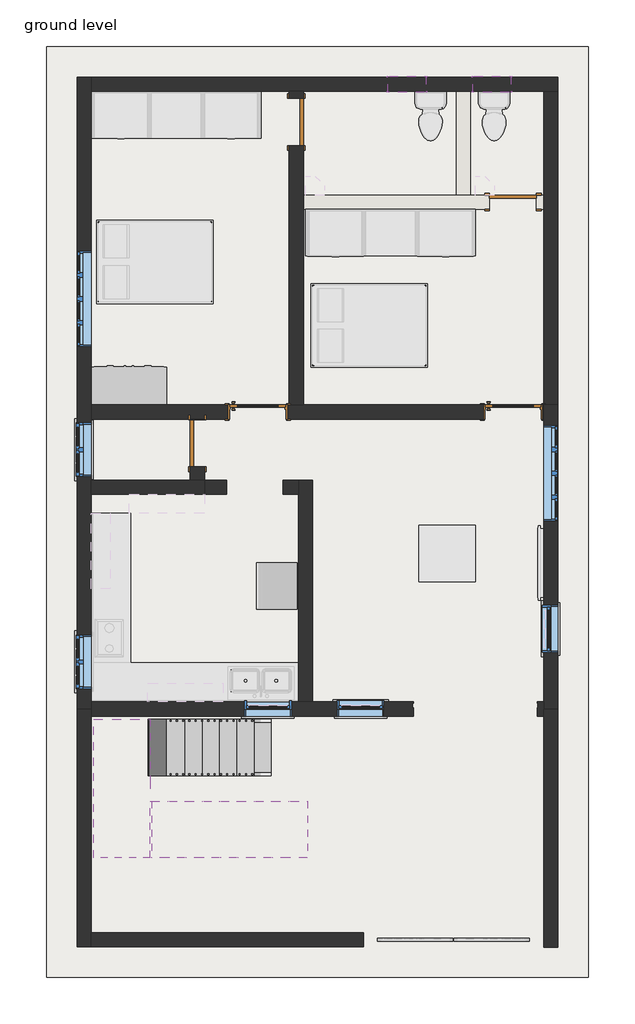
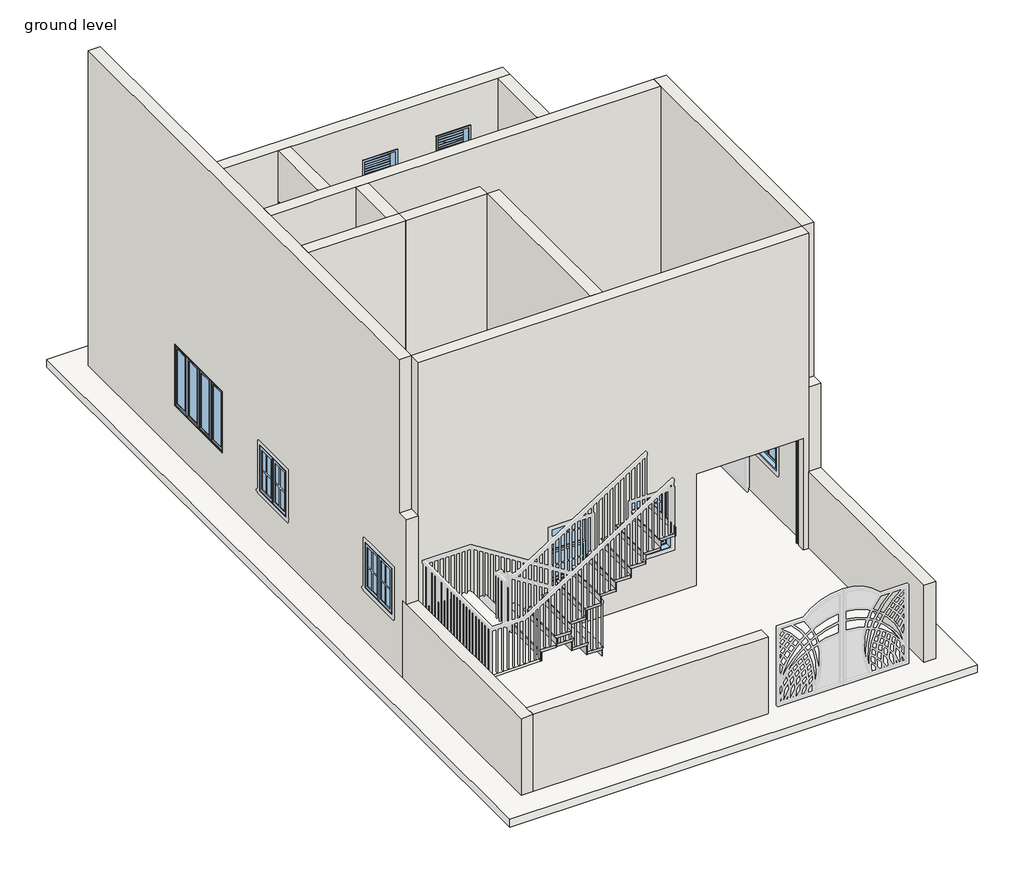
# One storey, part 1 of 3: 16 walls, 9 windows, 5 doors, 2 slabs, 2 stair flights.
"""IFC4 building model written with IfcOpenShell, lengths in millimetres."""

from ifc_helpers import new_model, si_unit, point, frame, origin, place, context, project, spatial, polyline, ellipse_curve, trimmed, outline, extrude, faceted_brep, transform, mapped, element, save
from ifc_brep_helpers import plane_surface, extruded_surface, advanced_brep
from components import door_3b97b8e7, door_bb98abfd, door_5e1232af, non_monolithic_landing_62f4187a, stair_flight_1669251e, stair_flight_fc52eaa6, window_339605e1, window_cf6260c5, window_d400040f, window_f2d8fef0

model = new_model("IFC4")

# Units and contexts
model_context = context("Model", 3, world=origin())
ifc_project = project(units=[si_unit("LENGTHUNIT", "METRE", prefix="MILLI")], contexts=[model_context])

# Site, building, storey
site = spatial("IfcSite", under=ifc_project)
building = spatial("IfcBuilding", under=site)
storey = spatial("IfcBuildingStorey", under=building, Name="ground level", Elevation=609.6)

# Doors
placement = place(None, origin())
door_shape = door_3b97b8e7(model_context)
element("IfcDoor", 1, ObjectType="Door-Interior-Single-1_Panel-Wood : 36\" x 84\"", at=placement, inside=storey, context=model_context, shape_type="MappedRepresentation", body=[
    mapped(door_shape, transform((31303.3316163, 14251.2730552, 609.6), x_axis=(1.0, 0.0, 0.0), y_axis=(0.0, 1.0, 0.0), z_axis=(0.0, 0.0, 1.0))),
])
element("IfcDoor", 2, ObjectType="Door-Interior-Single-1_Panel-Wood : 36\" x 84\"", at=placement, inside=storey, context=model_context, shape_type="MappedRepresentation", body=[
    mapped(door_shape, transform((35430.8316163, 14251.2730552, 609.6), x_axis=(1.0, 0.0, 0.0), y_axis=(0.0, 1.0, 0.0), z_axis=(0.0, 0.0, 1.0))),
])
door_2_shape = door_bb98abfd(model_context)
element("IfcDoor", 3, ObjectType="Single-Flush : 30\" x 84\"", at=placement, inside=storey, context=model_context, shape_type="MappedRepresentation", body=[
    mapped(door_2_shape, transform((30325.4316163, 13740.0980552, 609.6), x_axis=(0.0, 1.0, 0.0), y_axis=(-1.0, 0.0, 0.0), z_axis=(0.0, 0.0, 1.0))),
])
element("IfcDoor", 4, ObjectType="Single-Flush : 30\" x 84\"", at=placement, inside=storey, context=model_context, shape_type="MappedRepresentation", body=[
    mapped(door_2_shape, transform((35430.8316163, 17638.9980552, 609.6), x_axis=(1.0, 0.0, 0.0), y_axis=(0.0, 1.0, 0.0), z_axis=(0.0, 0.0, 1.0))),
])
door_3_shape = door_5e1232af(model_context)
element("IfcDoor", 5, ObjectType="Single-Flush : 30\" x 84\"", at=placement, inside=storey, context=model_context, shape_type="MappedRepresentation", body=[
    mapped(door_3_shape, transform((31925.6316163, 18934.3980552, 609.6), x_axis=(0.0, 1.0, 0.0), y_axis=(-1.0, 0.0, 0.0), z_axis=(0.0, 0.0, 1.0))),
])

# Slabs
element("IfcSlab", 6, ObjectType="Generic - 12\" 2", at=placement, inside=storey, context=model_context, shape_type="SweptSolid", body=[
    extrude(outline(polyline([(36650.0316163, 20153.5980552), (36650.0316163, 5110.4480552), (27887.0316163, 5110.4480552), (27887.0316163, 20153.5980552), (36650.0316163, 20153.5980552)])), frame((0.0, 0.0, 457.2), z_axis=(0.0, 0.0, 1.0), x_axis=(1.0, 0.0, 0.0)), (0.0, 0.0, 1.0), 152.4),
])
non_monolithic_landing_shape = non_monolithic_landing_62f4187a(model_context)
element("IfcSlab", 7, ObjectType="Non-Monolithic Landing", at=placement, inside=storey, context=model_context, shape_type="MappedRepresentation", body=[
    mapped(non_monolithic_landing_shape, transform((0.0, 0.0, 0.0), x_axis=(1.0, 0.0, 0.0), y_axis=(0.0, 1.0, 0.0), z_axis=(0.0, 0.0, 1.0))),
])

# Stair flights
stair_flight_shape = stair_flight_1669251e(model_context)
element("IfcStairFlight", 8, ObjectType="2\" Tread 1\" Nosing 1/4\" Riser", at=placement, inside=storey, context=model_context, shape_type="MappedRepresentation", body=[
    mapped(stair_flight_shape, transform((0.0, 0.0, 0.0), x_axis=(1.0, 0.0, 0.0), y_axis=(0.0, 1.0, 0.0), z_axis=(0.0, 0.0, 1.0))),
])
stair_flight_2_shape = stair_flight_fc52eaa6(model_context)
element("IfcStairFlight", 9, ObjectType="2\" Tread 1\" Nosing 1/4\" Riser", at=placement, inside=storey, context=model_context, shape_type="MappedRepresentation", body=[
    mapped(stair_flight_2_shape, transform((0.0, 0.0, 0.0), x_axis=(1.0, 0.0, 0.0), y_axis=(0.0, 1.0, 0.0), z_axis=(0.0, 0.0, 1.0))),
])

# Walls
element("IfcWall", 10, ObjectType="Generic - 9\"", at=placement, inside=storey, context=model_context, shape_type="Brep", body=[
    faceted_brep([(28610.9316163, 5605.7480552, 609.6), (28610.9316163, 5834.3480552, 609.6), (28610.9316163, 9333.1980552, 609.6), (28610.9316163, 9447.4980552, 609.6), (28610.9316163, 9447.4980552, 2133.6), (28610.9316163, 9333.1980552, 2133.6), (28610.9316163, 5834.3480552, 2133.6), (28610.9316163, 5605.7480552, 2133.6), (28382.3316163, 5605.7480552, 609.6), (28382.3316163, 5605.7480552, 2133.6), (28382.3316163, 9333.1980552, 2133.6), (28382.3316163, 9447.4980552, 2133.6), (28382.3316163, 9447.4980552, 609.6)], [[[0, 1, 2, 3, 4, 5, 6, 7]], [[8, 9, 10, 11, 12]], [[3, 2, 1, 0, 8, 12]], [[4, 3, 12, 11]], [[7, 6, 5, 4, 11, 10, 9]], [[0, 7, 9, 8]]]),
])
element("IfcWall", 11, ObjectType="Generic - 9\"", at=placement, inside=storey, context=model_context, shape_type="Brep", body=[
    faceted_brep([(28610.9316163, 14133.7980552, 609.6), (30211.1316163, 14133.7980552, 609.6), (30439.7316163, 14133.7980552, 609.6), (30820.7316163, 14133.7980552, 609.6), (30820.7316163, 14133.7980552, 2768.6), (31785.9316163, 14133.7980552, 2768.6), (31785.9316163, 14133.7980552, 609.6), (34948.2316163, 14133.7980552, 609.6), (34948.2316163, 14133.7980552, 2768.6), (35913.4316163, 14133.7980552, 2768.6), (35913.4316163, 14133.7980552, 609.6), (35926.1316163, 14133.7980552, 609.6), (35926.1316163, 14133.7980552, 6858.0), (30439.7316163, 14133.7980552, 6858.0), (30211.1316163, 14133.7980552, 6858.0), (28610.9316163, 14133.7980552, 6858.0), (30820.7316163, 14362.3980552, 609.6), (28610.9316163, 14362.3980552, 609.6), (28610.9316163, 14362.3980552, 6858.0), (32192.3316163, 14362.3980552, 6858.0), (35926.1316163, 14362.3980552, 6858.0), (35926.1316163, 14362.3980552, 3810.0), (35926.1316163, 14362.3980552, 609.6), (35913.4316163, 14362.3980552, 609.6), (35913.4316163, 14362.3980552, 2768.6), (34948.2316163, 14362.3980552, 2768.6), (34948.2316163, 14362.3980552, 609.6), (32039.9316163, 14362.3980552, 609.6), (31811.3316163, 14362.3980552, 609.6), (31785.9316163, 14362.3980552, 609.6), (31785.9316163, 14362.3980552, 2768.6), (30820.7316163, 14362.3980552, 2768.6)], [[[0, 1, 2, 3, 4, 5, 6, 7, 8, 9, 10, 11, 12, 13, 14, 15]], [[16, 17, 18, 19, 20, 21, 22, 23, 24, 25, 26, 27, 28, 29, 30, 31]], [[0, 17, 16, 3, 2, 1]], [[6, 29, 28, 27, 26, 7]], [[22, 11, 10, 23]], [[5, 30, 29, 6]], [[30, 5, 4, 31]], [[31, 4, 3, 16]], [[9, 24, 23, 10]], [[24, 9, 8, 25]], [[25, 8, 7, 26]], [[18, 15, 14, 13, 12, 20, 19]], [[15, 18, 17, 0]], [[11, 22, 21, 20, 12]]]),
])
element("IfcWall", 12, ObjectType="Generic - 9\"", at=placement, inside=storey, context=model_context, shape_type="Brep", body=[
    faceted_brep([(28610.9316163, 12914.5980552, 6858.0), (28610.9316163, 12914.5980552, 609.6), (30439.7316163, 12914.5980552, 609.6), (30439.7316163, 12914.5980552, 6858.0), (28610.9316163, 13143.1980552, 609.6), (28610.9316163, 13143.1980552, 6858.0), (30211.1316163, 13143.1980552, 6858.0), (30439.7316163, 13143.1980552, 6858.0), (30439.7316163, 13143.1980552, 609.6), (30211.1316163, 13143.1980552, 609.6)], [[[0, 1, 2, 3]], [[4, 5, 6, 7, 8, 9]], [[2, 1, 4, 9, 8]], [[0, 3, 7, 6, 5]], [[2, 8, 7, 3]], [[0, 5, 4, 1]]]),
])
element("IfcWall", 13, ObjectType="Generic - 9\"", at=placement, inside=storey, context=model_context, shape_type="SweptSolid", body=[
    extrude(outline(polyline([(14133.7980552, 609.6), (14121.0980552, 609.6), (14121.0980552, 2743.2), (13359.0980552, 2743.2), (13359.0980552, 609.6), (13143.1980552, 609.6), (13143.1980552, 6858.0), (14133.7980552, 6858.0), (14133.7980552, 609.6)])), frame((30211.1316163, 0.0, 0.0), z_axis=(1.0, 0.0, 0.0), x_axis=(0.0, 1.0, 0.0)), (0.0, 0.0, 1.0), 228.6),
])
element("IfcWall", 14, ObjectType="Generic - 9\"", at=placement, inside=storey, context=model_context, shape_type="Brep", body=[
    faceted_brep([(35926.1316163, 9333.1980552, 6858.0), (31519.2316163, 9333.1980552, 6858.0), (28610.9316163, 9333.1980552, 6858.0), (28610.9316163, 9333.1980552, 3810.0), (28610.9316163, 9333.1980552, 2133.6), (28610.9316163, 9333.1980552, 609.6), (33821.2316163, 9333.1980552, 609.6), (33821.2316163, 9333.1980552, 2818.6), (35821.2316163, 9333.1980552, 2818.6), (35821.2316163, 9333.1980552, 609.6), (35926.1316163, 9333.1980552, 609.6), (35926.1316163, 9333.1980552, 2133.6), (35926.1316163, 9333.1980552, 3810.0), (32586.0316163, 9333.1980552, 2692.4), (33348.0316163, 9333.1980552, 2692.4), (33348.0316163, 9333.1980552, 1524.0), (32586.0316163, 9333.1980552, 1524.0), (31087.4316163, 9333.1980552, 2692.4), (31849.4316163, 9333.1980552, 2692.4), (31849.4316163, 9333.1980552, 1524.0), (31087.4316163, 9333.1980552, 1524.0), (28610.9316163, 9561.7980552, 6858.0), (31963.7316163, 9561.7980552, 6858.0), (32192.3316163, 9561.7980552, 6858.0), (35926.1316163, 9561.7980552, 6858.0), (35926.1316163, 9561.7980552, 609.6), (35821.2316163, 9561.7980552, 609.6), (35821.2316163, 9561.7980552, 2818.6), (33821.2316163, 9561.7980552, 2818.6), (33821.2316163, 9561.7980552, 609.6), (32192.3316163, 9561.7980552, 609.6), (31963.7316163, 9561.7980552, 609.6), (28610.9316163, 9561.7980552, 609.6), (32586.0316163, 9561.7980552, 2692.4), (32586.0316163, 9561.7980552, 1524.0), (33348.0316163, 9561.7980552, 1524.0), (33348.0316163, 9561.7980552, 2692.4), (31087.4316163, 9561.7980552, 2692.4), (31087.4316163, 9561.7980552, 1524.0), (31849.4316163, 9561.7980552, 1524.0), (31849.4316163, 9561.7980552, 2692.4), (28610.9316163, 9447.4980552, 609.6), (33821.2316163, 9541.7980552, 609.6), (33806.2316163, 9541.7980552, 609.6), (33806.2316163, 9471.7980552, 609.6), (33821.2316163, 9471.7980552, 609.6), (35926.1316163, 9447.4980552, 609.6), (35821.2316163, 9471.7980552, 609.6), (35836.2316163, 9471.7980552, 609.6), (35836.2316163, 9541.7980552, 609.6), (35821.2316163, 9541.7980552, 609.6), (35821.2316163, 9541.7980552, 2818.6), (33821.2316163, 9541.7980552, 2818.6), (33821.2316163, 9471.7980552, 2818.6), (35821.2316163, 9471.7980552, 2818.6), (33806.2316163, 9471.7980552, 2833.6), (35836.2316163, 9471.7980552, 2833.6), (33806.2316163, 9541.7980552, 2833.6), (35836.2316163, 9541.7980552, 2833.6)], [[[0, 1, 2, 3, 4, 5, 6, 7, 8, 9, 10, 11, 12], [13, 14, 15, 16], [17, 18, 19, 20]], [[21, 22, 23, 24, 25, 26, 27, 28, 29, 30, 31, 32], [33, 34, 35, 36], [37, 38, 39, 40]], [[5, 41, 32, 31, 30, 29, 42, 43, 44, 45, 6]], [[25, 46, 10, 9, 47, 48, 49, 50, 26]], [[51, 52, 28, 27]], [[53, 54, 8, 7]], [[54, 47, 9, 8]], [[45, 53, 7, 6]], [[54, 53, 45, 44, 55, 56, 48, 47]], [[55, 44, 43, 57]], [[52, 51, 50, 49, 58, 57, 43, 42]], [[52, 42, 29, 28]], [[50, 51, 27, 26]], [[48, 56, 58, 49]], [[56, 55, 57, 58]], [[34, 33, 13, 16]], [[35, 34, 16, 15]], [[36, 35, 15, 14]], [[33, 36, 14, 13]], [[38, 37, 17, 20]], [[39, 38, 20, 19]], [[40, 39, 19, 18]], [[37, 40, 18, 17]], [[24, 23, 22, 21, 2, 1, 0]], [[10, 46, 25, 24, 0, 12, 11]], [[32, 41, 5, 4, 3, 2, 21]]]),
])
element("IfcWall", 15, ObjectType="Generic - 9\"", at=placement, inside=storey, context=model_context, shape_type="Brep", body=[
    faceted_brep([(32192.3316163, 9561.7980552, 6858.0), (32192.3316163, 9561.7980552, 609.6), (32192.3316163, 13143.1980552, 609.6), (32192.3316163, 13143.1980552, 3810.0), (32192.3316163, 12914.5980552, 3810.0), (32192.3316163, 12914.5980552, 6858.0), (31963.7316163, 9561.7980552, 609.6), (31963.7316163, 9561.7980552, 6858.0), (31963.7316163, 12914.5980552, 6858.0), (31963.7316163, 12914.5980552, 3810.0), (31963.7316163, 13143.1980552, 3810.0), (31963.7316163, 13143.1980552, 609.6), (31963.7316163, 12914.5980552, 609.6)], [[[0, 1, 2, 3, 4, 5]], [[6, 7, 8, 9, 10, 11, 12]], [[2, 1, 6, 12, 11]], [[0, 5, 8, 7]], [[0, 7, 6, 1]], [[9, 4, 3, 10]], [[3, 2, 11, 10]], [[5, 4, 9, 8]]]),
])
element("IfcWall", 16, ObjectType="Generic - 9\"", at=placement, inside=storey, context=model_context, shape_type="AdvancedBrep", body=[
    advanced_brep(
    [(30801.6816163, 13143.1980552, 2540.0), (30801.6816163, 13143.1980552, 609.6), (30439.7316163, 13143.1980552, 609.6), (30439.7316163, 13143.1980552, 6858.0), (31963.7316163, 13143.1980552, 6858.0), (31963.7316163, 13143.1980552, 3810.0), (31963.7316163, 13143.1980552, 609.6), (31716.0816163, 13143.1980552, 609.6), (31716.0816163, 13143.1980552, 2540.0), (30439.7316163, 12914.5980552, 609.6), (30801.6816163, 12914.5980552, 609.6), (30801.6816163, 12914.5980552, 2540.0), (31716.0816163, 12914.5980552, 2540.0), (31716.0816163, 12914.5980552, 609.6), (31963.7316163, 12914.5980552, 609.6), (31963.7316163, 12914.5980552, 6858.0), (30439.7316163, 12914.5980552, 6858.0)],
    [
        (0, 1),
        (1, 2),
        (2, 3),
        (3, 4),
        (4, 5),
        (5, 6),
        (6, 7),
        (7, 8),
        (8, 0, ellipse_curve(frame((31258.8816163, 13143.1980552, 2540.0), z_axis=(0.0, -1.0, 0.0), x_axis=(-1.0, 0.0, 0.0)), 457.2, 203.2)),
        (9, 10),
        (10, 11),
        (11, 12, ellipse_curve(frame((31258.8816163, 12914.5980552, 2540.0), z_axis=(0.0, 1.0, 0.0), x_axis=(-1.0, 0.0, 0.0)), 457.2, 203.2)),
        (12, 13),
        (13, 14),
        (14, 15),
        (15, 16),
        (16, 9),
        (6, 14),
        (13, 7),
        (1, 10),
        (9, 2),
        (11, 0),
        (8, 12),
        (3, 16),
        (15, 4),
    ],
    [
        plane_surface(frame((31963.7316163, 13143.1980552, 609.6), z_axis=(0.0, 1.0, 0.0), x_axis=(-1.0, 0.0, 0.0))),
        plane_surface(frame((31963.7316163, 12914.5980552, 609.6), z_axis=(0.0, -1.0, 0.0), x_axis=(1.0, 0.0, 0.0))),
        plane_surface(frame((32078.0316163, 13143.1980552, 609.6), z_axis=(0.0, 0.0, -1.0), x_axis=(0.0, -1.0, 0.0))),
        extruded_surface(trimmed(ellipse_curve(frame((31258.8816163, 13371.7980552, 2540.0), z_axis=(0.0, 1.0, 0.0), x_axis=(-1.0, 0.0, 0.0)), 457.2, 203.2), [point((30801.6816163, 13371.7980552, 2540.0))], [point((31716.0816163, 13371.7980552, 2540.0))], True, "CARTESIAN"), (0.0, -228.60000000000036, 0.0), 228.60000000000036),
        plane_surface(frame((31716.0816163, 12914.5980552, 2540.0), z_axis=(-1.0, 0.0, 0.0), x_axis=(0.0, 1.0, 0.0))),
        plane_surface(frame((30801.6816163, 12914.5980552, 609.6), z_axis=(1.0, 0.0, 0.0), x_axis=(0.0, 1.0, 0.0))),
        plane_surface(frame((32192.3316163, 19658.2980552, 6858.0), z_axis=(0.0, 0.0, 1.0), x_axis=(0.0, -1.0, 0.0))),
        plane_surface(frame((30439.7316163, 13028.8980552, 609.6), z_axis=(-1.0, 0.0, 0.0), x_axis=(0.0, 1.0, 0.0))),
        plane_surface(frame((31963.7316163, 9561.7980552, 609.6), z_axis=(1.0, 0.0, 0.0), x_axis=(0.0, -1.0, 0.0))),
    ],
    [
        (0, [[1, 2, 3, 4, 5, 6, 7, 8, 9]]),
        (1, [[10, 11, 12, 13, 14, 15, 16, 17]]),
        (2, [[-7, 18, -14, 19]]),
        (2, [[-2, 20, -10, 21]]),
        (3, [[-12, 22, -9, 23]]),
        (4, [[-13, -23, -8, -19]]),
        (5, [[-11, -20, -1, -22]]),
        (6, [[-4, 24, -16, 25]]),
        (7, [[-21, -17, -24, -3]]),
        (8, [[-25, -15, -18, -6, -5]]),
    ],
),
])
element("IfcWall", 17, ObjectType="Generic - 9\"", at=placement, inside=storey, context=model_context, shape_type="Brep", body=[
    faceted_brep([(28610.9316163, 9447.4980552, 609.6), (28610.9316163, 9561.7980552, 609.6), (28610.9316163, 12914.5980552, 609.6), (28610.9316163, 13143.1980552, 609.6), (28610.9316163, 14133.7980552, 609.6), (28610.9316163, 14362.3980552, 609.6), (28610.9316163, 19429.6980552, 609.6), (28610.9316163, 19658.2980552, 609.6), (28610.9316163, 19658.2980552, 3810.0), (28610.9316163, 19658.2980552, 6858.0), (28610.9316163, 19429.6980552, 6858.0), (28610.9316163, 14362.3980552, 6858.0), (28610.9316163, 14133.7980552, 6858.0), (28610.9316163, 13143.1980552, 6858.0), (28610.9316163, 12914.5980552, 6858.0), (28610.9316163, 9561.7980552, 6858.0), (28610.9316163, 9561.7980552, 3810.0), (28610.9316163, 9333.1980552, 3810.0), (28610.9316163, 9333.1980552, 2133.6), (28610.9316163, 9447.4980552, 2133.6), (28610.9316163, 16851.5980552, 2743.2), (28610.9316163, 16851.5980552, 1524.0), (28610.9316163, 15302.1980552, 1524.0), (28610.9316163, 15302.1980552, 2743.2), (28610.9316163, 14070.2980552, 2438.4), (28610.9316163, 14070.2980552, 1524.0), (28610.9316163, 13206.6980552, 1524.0), (28610.9316163, 13206.6980552, 2438.4), (28610.9316163, 10641.2980552, 2590.8), (28610.9316163, 10641.2980552, 1676.4), (28610.9316163, 9777.6980552, 1676.4), (28610.9316163, 9777.6980552, 2590.8), (28382.3316163, 9447.4980552, 609.6), (28382.3316163, 9447.4980552, 2133.6), (28382.3316163, 9333.1980552, 2133.6), (28382.3316163, 9333.1980552, 3810.0), (28382.3316163, 9561.7980552, 3810.0), (28382.3316163, 9561.7980552, 6858.0), (28382.3316163, 19429.6980552, 6858.0), (28382.3316163, 19658.2980552, 6858.0), (28382.3316163, 19658.2980552, 609.6), (28382.3316163, 16851.5980552, 2743.2), (28382.3316163, 15302.1980552, 2743.2), (28382.3316163, 15302.1980552, 1524.0), (28382.3316163, 16851.5980552, 1524.0), (28382.3316163, 14070.2980552, 2438.4), (28382.3316163, 13206.6980552, 2438.4), (28382.3316163, 13206.6980552, 1524.0), (28382.3316163, 14070.2980552, 1524.0), (28382.3316163, 10641.2980552, 2590.8), (28382.3316163, 9777.6980552, 2590.8), (28382.3316163, 9777.6980552, 1676.4), (28382.3316163, 10641.2980552, 1676.4)], [[[0, 1, 2, 3, 4, 5, 6, 7, 8, 9, 10, 11, 12, 13, 14, 15, 16, 17, 18, 19], [20, 21, 22, 23], [24, 25, 26, 27], [28, 29, 30, 31]], [[32, 33, 34, 35, 36, 37, 38, 39, 40], [41, 42, 43, 44], [45, 46, 47, 48], [49, 50, 51, 52]], [[7, 6, 5, 4, 3, 2, 1, 0, 32, 40]], [[21, 20, 41, 44]], [[22, 21, 44, 43]], [[23, 22, 43, 42]], [[20, 23, 42, 41]], [[25, 24, 45, 48]], [[26, 25, 48, 47]], [[27, 26, 47, 46]], [[24, 27, 46, 45]], [[29, 28, 49, 52]], [[30, 29, 52, 51]], [[31, 30, 51, 50]], [[28, 31, 50, 49]], [[15, 14, 13, 12, 11, 10, 9, 39, 38, 37]], [[0, 19, 33, 32]], [[18, 34, 33, 19]], [[16, 36, 35, 17]], [[18, 17, 35, 34]], [[15, 37, 36, 16]], [[7, 40, 39, 9, 8]]]),
])
element("IfcWall", 18, ObjectType="Generic - 9\"", at=placement, inside=storey, context=model_context, shape_type="Brep", body=[
    faceted_brep([(35926.1316163, 9447.4980552, 609.6), (35926.1316163, 9333.1980552, 609.6), (35926.1316163, 5599.3980552, 609.6), (35926.1316163, 5599.3980552, 2133.6), (35926.1316163, 9333.1980552, 2133.6), (35926.1316163, 9447.4980552, 2133.6), (36154.7316163, 9447.4980552, 609.6), (36154.7316163, 9447.4980552, 2133.6), (36154.7316163, 9333.1980552, 2133.6), (36154.7316163, 5599.3980552, 2133.6), (36154.7316163, 5599.3980552, 609.6)], [[[0, 1, 2, 3, 4, 5]], [[6, 7, 8, 9, 10]], [[2, 1, 0, 6, 10]], [[3, 2, 10, 9]], [[5, 4, 3, 9, 8, 7]], [[0, 5, 7, 6]]]),
])
element("IfcWall", 19, ObjectType="Generic - 9\"", at=placement, inside=storey, context=model_context, shape_type="SweptSolid", body=[
    extrude(outline(polyline([(33011.4468179, 5605.7480552), (28610.9316163, 5605.7480552), (28610.9316163, 5834.3480552), (33011.4468179, 5834.3480552), (33011.4468179, 5605.7480552)])), frame((0.0, 0.0, 609.6), z_axis=(0.0, 0.0, 1.0), x_axis=(1.0, 0.0, 0.0)), (0.0, 0.0, 1.0), 1524.0),
])
element("IfcWall", 20, ObjectType="Generic - 9\"", at=placement, inside=storey, context=model_context, shape_type="Brep", body=[
    faceted_brep([(35926.1316163, 14362.3980552, 6858.0), (35926.1316163, 14362.3980552, 4114.8), (35926.1316163, 14362.3980552, 3810.0), (35926.1316163, 14362.3980552, 609.6), (35926.1316163, 14133.7980552, 609.6), (35926.1316163, 9561.7980552, 609.6), (35926.1316163, 9447.4980552, 609.6), (35926.1316163, 9447.4980552, 2133.6), (35926.1316163, 9333.1980552, 2133.6), (35926.1316163, 9333.1980552, 3810.0), (35926.1316163, 9561.7980552, 3810.0), (35926.1316163, 9561.7980552, 6858.0), (35926.1316163, 14133.7980552, 6858.0), (35926.1316163, 12482.7980552, 2743.2), (35926.1316163, 12482.7980552, 1524.0), (35926.1316163, 14032.1980552, 1524.0), (35926.1316163, 14032.1980552, 2743.2), (35926.1316163, 10361.8980552, 2692.4), (35926.1316163, 10361.8980552, 1524.0), (35926.1316163, 11123.8980552, 1524.0), (35926.1316163, 11123.8980552, 2692.4), (36154.7316163, 14362.3980552, 609.6), (36154.7316163, 14362.3980552, 3810.0), (36154.7316163, 14362.3980552, 4114.8), (36154.7316163, 14362.3980552, 6858.0), (36154.7316163, 9561.7980552, 6858.0), (36154.7316163, 9561.7980552, 3810.0), (36154.7316163, 9333.1980552, 3810.0), (36154.7316163, 9333.1980552, 2133.6), (36154.7316163, 9447.4980552, 2133.6), (36154.7316163, 9447.4980552, 609.6), (36154.7316163, 12482.7980552, 2743.2), (36154.7316163, 14032.1980552, 2743.2), (36154.7316163, 14032.1980552, 1524.0), (36154.7316163, 12482.7980552, 1524.0), (36154.7316163, 10361.8980552, 2692.4), (36154.7316163, 11123.8980552, 2692.4), (36154.7316163, 11123.8980552, 1524.0), (36154.7316163, 10361.8980552, 1524.0)], [[[0, 1, 2, 3, 4, 5, 6, 7, 8, 9, 10, 11, 12], [13, 14, 15, 16], [17, 18, 19, 20]], [[21, 22, 23, 24, 25, 26, 27, 28, 29, 30], [31, 32, 33, 34], [35, 36, 37, 38]], [[6, 5, 4, 3, 21, 30]], [[7, 6, 30, 29]], [[28, 8, 7, 29]], [[26, 10, 9, 27]], [[9, 8, 28, 27]], [[10, 26, 25, 11]], [[13, 16, 32, 31]], [[16, 15, 33, 32]], [[15, 14, 34, 33]], [[14, 13, 31, 34]], [[17, 20, 36, 35]], [[20, 19, 37, 36]], [[19, 18, 38, 37]], [[18, 17, 35, 38]], [[0, 12, 11, 25, 24]], [[0, 24, 23, 22, 21, 3, 2, 1]]]),
])
element("IfcWall", 21, ObjectType="Generic - 9\"", at=placement, inside=storey, context=model_context, shape_type="Brep", body=[
    faceted_brep([(31811.3316163, 19429.6980552, 609.6), (31811.3316163, 19315.3980552, 609.6), (31811.3316163, 19315.3980552, 2743.2), (31811.3316163, 18553.3980552, 2743.2), (31811.3316163, 18553.3980552, 609.6), (31811.3316163, 14362.3980552, 609.6), (31811.3316163, 14362.3980552, 3810.0), (31811.3316163, 19429.6980552, 3810.0), (32039.9316163, 19315.3980552, 2743.2), (32039.9316163, 19315.3980552, 609.6), (32039.9316163, 19429.6980552, 609.6), (32039.9316163, 19429.6980552, 3810.0), (32039.9316163, 14362.3980552, 3810.0), (32039.9316163, 14362.3980552, 609.6), (32039.9316163, 17524.6980552, 609.6), (32039.9316163, 17753.2980552, 609.6), (32039.9316163, 18553.3980552, 609.6), (32039.9316163, 18553.3980552, 2743.2)], [[[0, 1, 2, 3, 4, 5, 6, 7]], [[8, 9, 10, 11, 12, 13, 14, 15, 16, 17]], [[10, 9, 1, 0]], [[16, 15, 14, 13, 5, 4]], [[7, 6, 12, 11]], [[6, 5, 13, 12]], [[0, 7, 11, 10]], [[2, 1, 9, 8]], [[3, 2, 8, 17]], [[4, 3, 17, 16]]]),
])
element("IfcWall", 22, ObjectType="Generic - 9\"", at=placement, inside=storey, context=model_context, shape_type="Brep", body=[
    faceted_brep([(28610.9316163, 19429.6980552, 609.6), (31811.3316163, 19429.6980552, 609.6), (32039.9316163, 19429.6980552, 609.6), (34516.4316163, 19429.6980552, 609.6), (34745.0316163, 19429.6980552, 609.6), (35926.1316163, 19429.6980552, 609.6), (36154.7316163, 19429.6980552, 609.6), (36154.7316163, 19429.6980552, 3810.0), (35926.1316163, 19429.6980552, 3810.0), (32192.3316163, 19429.6980552, 3810.0), (32039.9316163, 19429.6980552, 3810.0), (31811.3316163, 19429.6980552, 3810.0), (28610.9316163, 19429.6980552, 3810.0), (33411.5316163, 19429.6980552, 3048.0), (34021.1316163, 19429.6980552, 3048.0), (34021.1316163, 19429.6980552, 2438.4), (33411.5316163, 19429.6980552, 2438.4), (34783.1316163, 19429.6980552, 3048.0), (35392.7316163, 19429.6980552, 3048.0), (35392.7316163, 19429.6980552, 2438.4), (34783.1316163, 19429.6980552, 2438.4), (28610.9316163, 19658.2980552, 609.6), (28610.9316163, 19658.2980552, 3810.0), (32192.3316163, 19658.2980552, 3810.0), (36154.7316163, 19658.2980552, 3810.0), (36154.7316163, 19658.2980552, 609.6), (33411.5316163, 19658.2980552, 3048.0), (33411.5316163, 19658.2980552, 2438.4), (34021.1316163, 19658.2980552, 2438.4), (34021.1316163, 19658.2980552, 3048.0), (34783.1316163, 19658.2980552, 3048.0), (34783.1316163, 19658.2980552, 2438.4), (35392.7316163, 19658.2980552, 2438.4), (35392.7316163, 19658.2980552, 3048.0)], [[[0, 1, 2, 3, 4, 5, 6, 7, 8, 9, 10, 11, 12], [13, 14, 15, 16], [17, 18, 19, 20]], [[21, 22, 23, 24, 25], [26, 27, 28, 29], [30, 31, 32, 33]], [[6, 5, 4, 3, 2, 1, 0, 21, 25]], [[12, 11, 10, 9, 8, 7, 24, 23, 22]], [[0, 12, 22, 21]], [[7, 6, 25, 24]], [[27, 26, 13, 16]], [[28, 27, 16, 15]], [[29, 28, 15, 14]], [[26, 29, 14, 13]], [[31, 30, 17, 20]], [[32, 31, 20, 19]], [[33, 32, 19, 18]], [[30, 33, 18, 17]]]),
])
element("IfcWall", 23, ObjectType="Generic - 9\"", at=placement, inside=storey, context=model_context, shape_type="Brep", body=[
    faceted_brep([(35926.1316163, 19429.6980552, 609.6), (35926.1316163, 17753.2980552, 609.6), (35926.1316163, 17524.6980552, 609.6), (35926.1316163, 14362.3980552, 609.6), (35926.1316163, 14362.3980552, 3810.0), (35926.1316163, 19429.6980552, 3810.0), (36154.7316163, 19429.6980552, 609.6), (36154.7316163, 19429.6980552, 3810.0), (36154.7316163, 14362.3980552, 3810.0), (36154.7316163, 14362.3980552, 609.6)], [[[0, 1, 2, 3, 4, 5]], [[6, 7, 8, 9]], [[3, 2, 1, 0, 6, 9]], [[5, 4, 8, 7]], [[0, 5, 7, 6]], [[4, 3, 9, 8]]]),
])
element("IfcWall", 24, ObjectType="Generic - 9\"", at=placement, inside=storey, context=model_context, shape_type="Brep", body=[
    faceted_brep([(35926.1316163, 17524.6980552, 609.6), (35926.1316163, 17524.6980552, 914.4), (35811.8316163, 17524.6980552, 914.4), (35811.8316163, 17524.6980552, 609.6), (35926.1316163, 17753.2980552, 914.4), (35926.1316163, 17753.2980552, 609.6), (35811.8316163, 17753.2980552, 609.6), (35811.8316163, 17753.2980552, 914.4)], [[[0, 1, 2, 3]], [[4, 5, 6, 7]], [[5, 0, 3, 6]], [[1, 4, 7, 2]], [[1, 0, 5, 4]], [[3, 2, 7, 6]]]),
    faceted_brep([(32039.9316163, 17524.6980552, 914.4), (32039.9316163, 17524.6980552, 609.6), (35049.8316163, 17524.6980552, 609.6), (35049.8316163, 17524.6980552, 914.4), (32039.9316163, 17753.2980552, 609.6), (32039.9316163, 17753.2980552, 914.4), (34516.4316163, 17753.2980552, 914.4), (34745.0316163, 17753.2980552, 914.4), (35049.8316163, 17753.2980552, 914.4), (35049.8316163, 17753.2980552, 609.6), (34745.0316163, 17753.2980552, 609.6), (34516.4316163, 17753.2980552, 609.6)], [[[0, 1, 2, 3]], [[4, 5, 6, 7, 8, 9, 10, 11]], [[1, 4, 11, 10, 9, 2]], [[5, 0, 3, 8, 7, 6]], [[1, 0, 5, 4]], [[3, 2, 9, 8]]]),
])
element("IfcWall", 25, ObjectType="Generic - 9\"", at=placement, inside=storey, context=model_context, shape_type="SweptSolid", body=[
    extrude(outline(polyline([(34516.4316163, 17753.2980552), (34516.4316163, 19429.6980552), (34745.0316163, 19429.6980552), (34745.0316163, 17753.2980552), (34516.4316163, 17753.2980552)])), frame((0.0, 0.0, 609.6), z_axis=(0.0, 0.0, 1.0), x_axis=(1.0, 0.0, 0.0)), (0.0, 0.0, 1.0), 304.8),
])

# Windows
window_shape = window_339605e1(model_context)
element("IfcWindow", 26, ObjectType="Window-Casement-Double : 34\" x 36\"", at=placement, inside=storey, context=model_context, shape_type="MappedRepresentation", body=[
    mapped(window_shape, transform((28496.6316163, 13638.4980552, 609.6), x_axis=(0.0, 1.0, 0.0), y_axis=(-1.0, 0.0, 0.0), z_axis=(0.0, 0.0, 1.0))),
])
element("IfcWindow", 27, ObjectType="Window-Casement-Double : 34\" x 36\"", at=placement, inside=storey, context=model_context, shape_type="MappedRepresentation", body=[
    mapped(window_shape, transform((28496.6316163, 10209.4980552, 762.0), x_axis=(0.0, 1.0, 0.0), y_axis=(-1.0, 0.0, 0.0), z_axis=(0.0, 0.0, 1.0))),
])
window_2_shape = window_cf6260c5(model_context)
element("IfcWindow", 28, ObjectType="Window-Casement-Multi-Sash-Horizontal : 61\" x 48\"", at=placement, inside=storey, context=model_context, shape_type="MappedRepresentation", body=[
    mapped(window_2_shape, transform((28496.6316163, 16076.8980552, 609.6), x_axis=(0.0, 1.0, 0.0), y_axis=(-1.0, 0.0, 0.0), z_axis=(0.0, 0.0, 1.0))),
])
element("IfcWindow", 29, ObjectType="Window-Casement-Multi-Sash-Horizontal : 61\" x 48\"", at=placement, inside=storey, context=model_context, shape_type="MappedRepresentation", body=[
    mapped(window_2_shape, transform((36040.4316163, 13257.4980552, 609.6), x_axis=(0.0, -1.0, 0.0), y_axis=(1.0, 0.0, 0.0), z_axis=(0.0, 0.0, 1.0))),
])
window_3_shape = window_d400040f(model_context)
element("IfcWindow", 30, ObjectType="Window-Double-Hung : 30\" x 46\"", at=placement, inside=storey, context=model_context, shape_type="MappedRepresentation", body=[
    mapped(window_3_shape, transform((32967.0316163, 9447.4980552, 609.6), x_axis=(1.0, 0.0, 0.0), y_axis=(0.0, 1.0, 0.0), z_axis=(0.0, 0.0, 1.0))),
])
element("IfcWindow", 31, ObjectType="Window-Double-Hung : 30\" x 46\"", at=placement, inside=storey, context=model_context, shape_type="MappedRepresentation", body=[
    mapped(window_3_shape, transform((36040.4316163, 10742.8980552, 609.6), x_axis=(0.0, 1.0, 0.0), y_axis=(-1.0, 0.0, 0.0), z_axis=(0.0, 0.0, 1.0))),
])
element("IfcWindow", 32, ObjectType="Window-Double-Hung : 30\" x 46\"", at=placement, inside=storey, context=model_context, shape_type="MappedRepresentation", body=[
    mapped(window_3_shape, transform((31468.4316163, 9447.4980552, 609.6), x_axis=(1.0, 0.0, 0.0), y_axis=(0.0, 1.0, 0.0), z_axis=(0.0, 0.0, 1.0))),
])
window_4_shape = window_f2d8fef0(model_context)
element("IfcWindow", 33, ObjectType="Window-Louvers : 24\" x 24\"", at=placement, inside=storey, context=model_context, shape_type="MappedRepresentation", body=[
    mapped(window_4_shape, transform((33716.3316163, 19550.3480552, 1524.0), x_axis=(1.0, 0.0, 0.0), y_axis=(0.0, 1.0, 0.0), z_axis=(0.0, 0.0, 1.0))),
])
element("IfcWindow", 34, ObjectType="Window-Louvers : 24\" x 24\"", at=placement, inside=storey, context=model_context, shape_type="MappedRepresentation", body=[
    mapped(window_4_shape, transform((35087.9316163, 19550.3480552, 1524.0), x_axis=(1.0, 0.0, 0.0), y_axis=(0.0, 1.0, 0.0), z_axis=(0.0, 0.0, 1.0))),
])

save(model, "model.ifc")

# Revit data of these elements
# Type "Door-Interior-Single-1_Panel-Wood : 36\" x 84\""
#   Type Mark = "8"
#   Assembly Code = "C1020300"
#   Analytic Construction = "Wooden"
#   Top Rail = 0' - 4 11/16"
#   Thickness = 0' - 1 3/8"
#   Thermal Resistance (R) = 2.5876 (h·ft²·°F)/BTU
#   Swing Angle [instance default] = 90.00°
#   Stiles = 0' - 4 3/4"
#   Rough Width = 3' - 2"
#   Rough Height = 7' - 1"
#   Height = 7' - 0"
#   Width = 3' - 0"
#   Heat Transfer Coefficient (U) = 0.3865 BTU/(h·ft²·°F)
#   Bottom Rail = 0' - 9 1/8"
#   Trim Material = Cherry
#   Panel Material = Cherry
#   Frame Material = Cherry
#   Door Handle Material = Aluminum
#   Visual Light Transmittance = 0
#   Solar Heat Gain Coefficient = 0
#   Wall Closure = (empty or 0)
#   Function = (empty or 0)
# Type "Single-Flush : 30\" x 84\""
#   Type Mark = "4"
#   Construction Type Id = "MDOOR"
#   Assembly Code = "C1020"
#   Analytic Construction = "Metal"
#   Thickness = 0' - 2"
#   Heat Transfer Coefficient (U) = 0.651978 BTU/(h·ft²·°F)
#   Height = 7' - 0"
#   Trim Projection Ext = 0' - 1"
#   Trim Projection Int = 0' - 1"
#   Trim Width = 0' - 3"
#   Width = 2' - 6"
#   Define Thermal Properties by = 1
#   Define Thermal Properties by = 1
#   Door Material = Door - Panel
#   Frame Material = Door - Frame
#   Visual Light Transmittance = 0
#   Solar Heat Gain Coefficient = 0
#   Function = (empty or 0)
#   Wall Closure = (empty or 0)
# Type "Generic - 12\" 2"
#   Assembly Code = "B1010"
#   Function = 0
#   Layers, outside or top first: 0' - 6" no material (function 1)
# Type "Generic - 9\""
#   Assembly Code = "B2010"
#   Layers, outside or top first: 0' - 9" no material (function 1)
# Type "Window-Casement-Double : 34\" x 36\""
#   Type Mark = "14"
#   Fire Rating = "0.5h"
#   Assembly Code = "B2020100"
#   Analytic Construction = "Double glazing - domestic"
#   Frame Extension [instance default] = 0' - 0 1/4"
#   Window Inset [instance default] = 0' - 0"
#   Wall Thickness [instance default] = 0' - 6"
#   Interior Wall Closure [instance default] = 0' - 2 1/4"
#   Half Width = 1' - 5"
#   Visual Light Transmittance = 0.81
#   Thermal Resistance (R) = 1.8146 (h·ft²·°F)/BTU
#   Solar Heat Gain Coefficient = 0.76
#   Rough Width = 2' - 10 1/2"
#   Rough Height = 3' - 0 1/2"
#   Height = 3' - 0"
#   Heat Transfer Coefficient (U) = 0.5511 BTU/(h·ft²·°F)
#   Exterior Wall Closure [instance default] = 0' - 1 1/4"
#   Extension Jamb [instance default] = 0' - 2 1/4"
#   Default Sill Height = 3' - 0"
#   Width = 2' - 10"
#   Define Thermal Properties by = 0
#   Muntin Visibility = yes
#   Interior Trim Visibility [instance default] = yes
#   Exterior Trim Visibility [instance default] = yes
#   Extension Jamb Visibility [instance default] = yes
#   Interior Trim Material = Wood - Stained
#   Muntin Pattern = Muntin Pattern_2x2 : Muntin Pattern_2x2
#   Interior Trim = Trim-Window-Interior-Flat : Picture Frame
#   Interior Frame Material = Wood - Stained
#   Glass Panel Material = Glass
#   Exterior Trim Material = Clad - White
#   Exterior Trim = Trim-Window-Exterior-Flat : with Sill
#   Exterior Frame Material = Clad - White
#   Wall Closure = (empty or 0)
# Type "Window-Casement-Multi-Sash-Horizontal : 61\" x 48\""
#   Type Mark = "21"
#   Fire Rating = "0.5h"
#   Assembly Code = "B2020100"
#   Analytic Construction = "Double glazing - domestic"
#   Window Inset [instance default] = 0' - 0 5/8"
#   Wall Thickness [instance default] = 0' - 6"
#   Visual Light Transmittance = 0.81
#   Thermal Resistance (R) = 1.8146 (h·ft²·°F)/BTU
#   Solar Heat Gain Coefficient = 0.76
#   Rough Width = 5' - 1 1/2"
#   Rough Height = 4' - 0 1/2"
#   Open Window Width = 1' - 3 1/4"
#   Heat Transfer Coefficient (U) = 0.5511 BTU/(h·ft²·°F)
#   Height = 4' - 0"
#   Frame Gap 3 [instance default] = 0' - 1 83/128"
#   Frame Gap 2 [instance default] = 0' - 0 5/8"
#   Frame Gap 1 = 0' - 1 51/128"
#   Default Sill Height = 3' - 0"
#   Width = 5' - 1"
#   Frame Material = Metal - Aluminum
#   Glass Panel Material = Glass
#   Wall Closure = (empty or 0)
# Type "Window-Double-Hung : 30\" x 46\""
#   Type Mark = "13"
#   Fire Rating = "0.5h"
#   Construction Type Id = "DG-DR"
#   Assembly Code = "B2020100"
#   Analytic Construction = "Double glazing - domestic"
#   Wall Thickness [instance default] = 0' - 6"
#   Window Inset [instance default] = 0' - 0"
#   Visual Light Transmittance = 0.81
#   Thermal Resistance (R) = 1.8146 (h·ft²·°F)/BTU
#   Solar Heat Gain Coefficient = 0.76
#   Muntin Width = 2' - 0"
#   Muntin Height = 1' - 7 1/8"
#   Interior Wall Closure [instance default] = 0' - 1 1/2"
#   Rough Width = 2' - 6 1/2"
#   Rough Height = 3' - 10 1/2"
#   Frame Extension [instance default] = 0' - 1 1/4"
#   Exterior Wall Closure [instance default] = 0' - 0 1/2"
#   Extension Jamb [instance default] = 0' - 1 1/2"
#   Heat Transfer Coefficient (U) = 0.5511 BTU/(h·ft²·°F)
#   Height = 3' - 10"
#   Width = 2' - 6"
#   Define Thermal Properties by = 1
#   Top Muntin Visibility = yes
#   Indicator Visibility [instance default] = yes
#   Extension Jamb Visibility [instance default] = yes
#   Interior Trim Visibility [instance default] = yes
#   Exterior Trim Visibility [instance default] = yes
#   Define Thermal Properties by = 1
#   Bottom Muntin Visibility = yes
#   Muntin Pattern = Muntin Pattern_2x2 : Muntin Pattern_2x2
#   Interior Trim Material = Wood - Stained
#   Interior Trim = Trim-Window-Interior-Flat : Picture Frame
#   Exterior Trim Material = Clad - White
#   Exterior Trim = Trim-Window-Exterior-Flat : with Sill
#   Glass Panel Material = Glass
#   Exterior Frame Material = Clad - White
#   Interior Frame Material = Wood - Stained
#   Wall Closure = (empty or 0)
# Type "Window-Louvers : 24\" x 24\""
#   Type Mark = "18"
#   Construction Type Id = "GSP4R"
#   Assembly Code = "B20"
#   Analytic Construction = "1/8 in Pilkington single glazing"
#   Visual Light Transmittance = 0.9
#   Thermal Resistance (R) = 1.53941 (h·ft²·°F)/BTU
#   Solar Heat Gain Coefficient = 0.78
#   Max Height = 1' - 11.74264"
#   Height = 2' - 0"
#   Heat Transfer Coefficient (U) = 0.6496 BTU/(h·ft²·°F)
#   Blade Width [instance default] = 1' - 10 1/2"
#   Blade Vertical Thickness = 0' - 0.35355"
#   Blade Thickness = 0' - 0 1/4"
#   Blade Spacing = 0' - 1 1/2"
#   Blade Height = 0' - 1.85355"
#   Blade Depth = 0' - 3"
#   Blade Angle = 45.00°
#   Default Sill Height = 3' - 0"
#   Trim Projection_Exterior = 0' - 0 1/2"
#   Trim Projection_Interior = 0' - 0 1/2"
#   Trim Width_Exterior = 0' - 1 1/2"
#   Trim Width_Interior = 0' - 1 1/2"
#   Width = 2' - 0"
#   Max Blade Count = 12
#   Define Thermal Properties by = 1
#   Blade Count = 12
#   Frame Material = Birch
#   Louver Material = Birch
#   Trim Exterior Material = Birch
#   Trim Interior Material = Birch
#   Wall Closure = (empty or 0)
# Elements 1, 2 (IfcDoor, "Door-Interior-Single-1_Panel-Wood : 36\" x 84\"")
#   Swing Angle = 90.00°
#   Phase Created = New Construction
#   Materials on its faces: "Cherry", "Aluminum"
# Elements 3, 4, 5 (IfcDoor, "Single-Flush : 30\" x 84\"")
#   Phase Created = New Construction
#   Materials on its faces: "Door - Frame", "Door - Panel"
# Element 6 (IfcSlab, "Generic - 12\" 2")
#   Height Offset From Level = 0' - 0"
#   Phase Created = New Construction
#   Materials on its faces: "Default Floor"
# Element 7 (IfcSlab, "Non-Monolithic Landing")
#   Phase Created = New Construction
# Elements 8, 9 (IfcStairFlight, "2\" Tread 1\" Nosing 1/4\" Riser")
#   Phase Created = New Construction
# Elements 10, 18, 19 (IfcWall, "Generic - 9\"")
#   Top Offset = 0' - 0"
#   Base Offset = 0' - 0"
#   Unconnected Height = 5' - 0"
#   wall height = 5' - 0"
#   Phase Created = New Construction
#   Base Constraint = ground level
#   Materials on its faces: "Default Wall"
# Elements 11, 12, 13, 14, 15, 16, 17, 20 (IfcWall, "Generic - 9\"")
#   Top Offset = 0' - 0"
#   Base Offset = 0' - 0"
#   wall height = 20' - 6"
#   Phase Created = New Construction
#   Base Constraint = ground level
#   Top Constraint = 1st floor
#   Materials on its faces: "Default Wall"
# Elements 21, 22, 23 (IfcWall, "Generic - 9\"")
#   Top Offset = 0' - 0"
#   Base Offset = 0' - 0"
#   wall height = 10' - 6"
#   Phase Created = New Construction
#   Base Constraint = ground level
#   Top Constraint = 1st floor
#   Materials on its faces: "Default Wall"
# Elements 24, 25 (IfcWall, "Generic - 9\"")
#   Top Offset = 0' - 0"
#   Base Offset = 0' - 0"
#   Unconnected Height = 1' - 0"
#   wall height = 1' - 0"
#   Phase Created = New Construction
#   Base Constraint = ground level
#   Materials on its faces: "Default Wall"
# Element 26 (IfcWindow, "Window-Casement-Double : 34\" x 36\"")
#   Mark = "25"
#   Window Inset = 0' - 0"
#   Interior Wall Closure = 0' - 2 1/4"
#   Frame Extension = 0' - 0 1/4"
#   Exterior Wall Closure = 0' - 1 1/4"
#   Interior Trim Visibility = yes
#   Exterior Trim Visibility = yes
#   Phase Created = New Construction
#   Materials on its faces: "Wood - Stained", "Glass", "Clad - White"
# Element 27 (IfcWindow, "Window-Casement-Double : 34\" x 36\"")
#   Mark = "26"
#   Window Inset = 0' - 0"
#   Interior Wall Closure = 0' - 2 1/4"
#   Frame Extension = 0' - 0 1/4"
#   Exterior Wall Closure = 0' - 1 1/4"
#   Interior Trim Visibility = yes
#   Exterior Trim Visibility = yes
#   Phase Created = New Construction
#   Materials on its faces: "Wood - Stained", "Glass", "Clad - White"
# Element 28 (IfcWindow, "Window-Casement-Multi-Sash-Horizontal : 61\" x 48\"")
#   Mark = "22"
#   Window Inset = 0' - 0 5/8"
#   Frame Gap 3 = 0' - 1 83/128"
#   Frame Gap 2 = 0' - 0 5/8"
#   Phase Created = New Construction
#   Materials on its faces: "Metal - Aluminum", "Glass"
# Element 29 (IfcWindow, "Window-Casement-Multi-Sash-Horizontal : 61\" x 48\"")
#   Mark = "24"
#   Window Inset = 0' - 0 5/8"
#   Frame Gap 3 = 0' - 1 83/128"
#   Frame Gap 2 = 0' - 0 5/8"
#   Phase Created = New Construction
#   Materials on its faces: "Metal - Aluminum", "Glass"
# Element 30 (IfcWindow, "Window-Double-Hung : 30\" x 46\"")
#   Mark = "27"
#   Window Inset = 0' - 0"
#   Interior Wall Closure = 0' - 1 1/2"
#   Frame Extension = 0' - 1 1/4"
#   Exterior Wall Closure = 0' - 0 1/2"
#   Interior Trim Visibility = yes
#   Indicator Visibility = yes
#   Exterior Trim Visibility = yes
#   Phase Created = New Construction
#   Materials on its faces: "Wood - Stained", "Glass", "Clad - White"
# Element 31 (IfcWindow, "Window-Double-Hung : 30\" x 46\"")
#   Mark = "28"
#   Window Inset = 0' - 0"
#   Interior Wall Closure = 0' - 1 1/2"
#   Frame Extension = 0' - 1 1/4"
#   Exterior Wall Closure = 0' - 0 1/2"
#   Interior Trim Visibility = yes
#   Indicator Visibility = yes
#   Exterior Trim Visibility = yes
#   Phase Created = New Construction
#   Materials on its faces: "Wood - Stained", "Glass", "Clad - White"
# Element 32 (IfcWindow, "Window-Double-Hung : 30\" x 46\"")
#   Mark = "30"
#   Window Inset = 0' - 0"
#   Interior Wall Closure = 0' - 1 1/2"
#   Frame Extension = 0' - 1 1/4"
#   Exterior Wall Closure = 0' - 0 1/2"
#   Interior Trim Visibility = yes
#   Indicator Visibility = yes
#   Exterior Trim Visibility = yes
#   Phase Created = New Construction
#   Materials on its faces: "Wood - Stained", "Glass", "Clad - White"
# Element 33 (IfcWindow, "Window-Louvers : 24\" x 24\"")
#   Mark = "51"
#   Blade Width = 1' - 10 1/2"
#   Phase Created = New Construction
#   Materials on its faces: "Birch"
# Element 34 (IfcWindow, "Window-Louvers : 24\" x 24\"")
#   Mark = "52"
#   Blade Width = 1' - 10 1/2"
#   Phase Created = New Construction
#   Materials on its faces: "Birch"
# Materials
#   "Cherry": class "Wood", colour RGB 226 177 128, transparency 0, Description = "Prunus Serotina", Cost = 0
#   "Aluminum": class "Metal", colour RGB 247 247 247, transparency 0, Description = "Aluminum 6061", Cost = 0
#   "Door - Panel": class "Wood", colour RGB 210 159 95, transparency 0, Cost = 0
#   "Door - Frame": colour RGB 118 70 51, transparency 0, Cost = 0
#   "Wood - Stained": class "Wood", colour RGB 224 178 126, transparency 0, Cost = 0
#   "Glass": class "Glass", colour RGB 0 128 192, transparency 0.75, Description = "Soda Lime Glass", Cost = 0
#   "Clad - White": class "Wood", colour RGB 242 242 238, transparency 0, Cost = 0
#   "Metal - Aluminum": class "Metal", colour RGB 247 247 247, transparency 0
#   "Birch": class "Wood", colour RGB 224 178 126, transparency 0, Description = "Betula Alleghaniensis", Cost = 0
#   "Default Floor": colour RGB 128 128 128, transparency 0, Cost = 0
#   "Default Wall": colour RGB 128 128 128, transparency 0, Cost = 0
